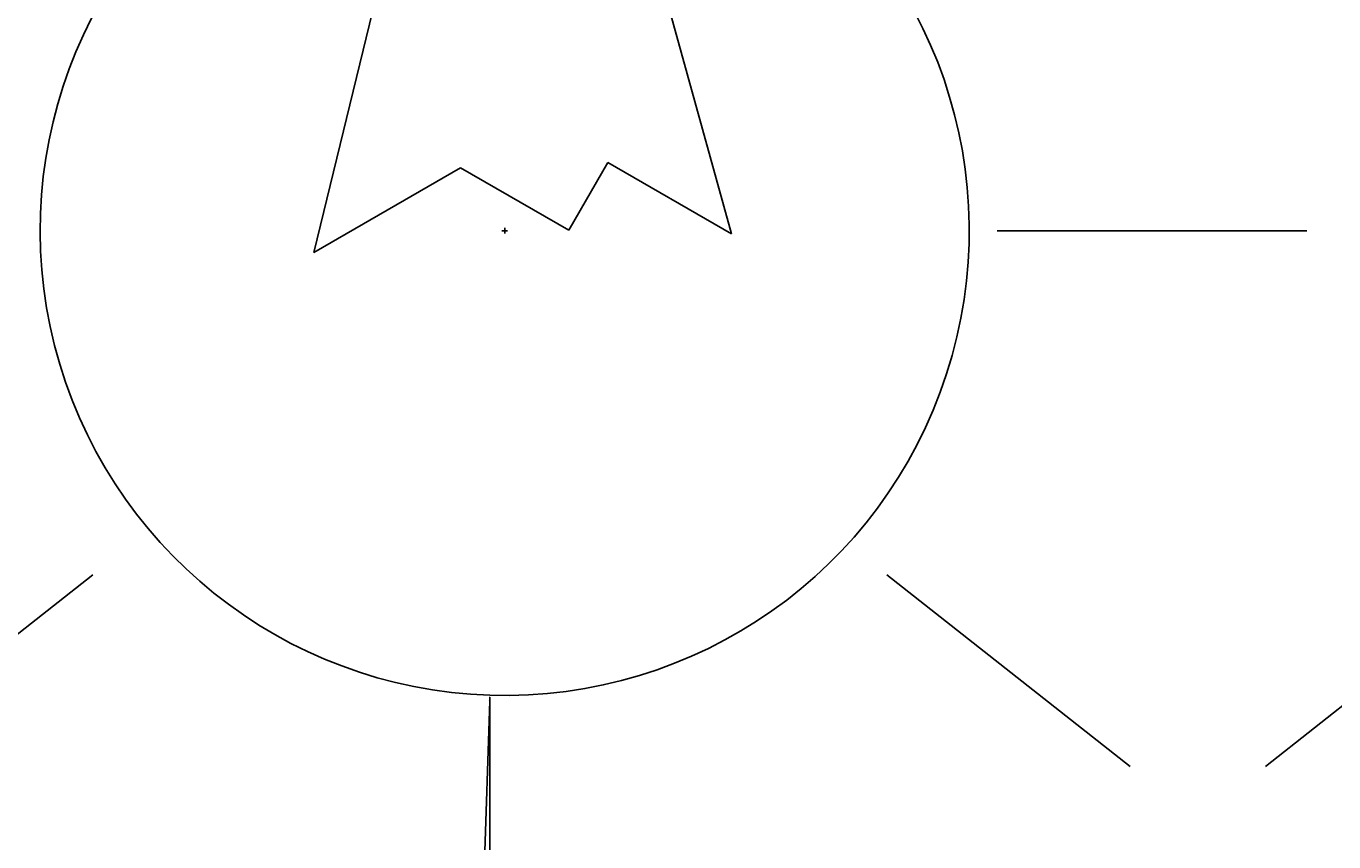
# Model space of a CAD drawing. Units: millimetres. Extents: x -8 to 285, y 5 to 221.
# Tile 23 of 30: x 130 to 172, y 132 to 159. Entities that reach past the tile are written whole.
import ezdxf

# ---------------------------------------------------------------- set-up
doc = ezdxf.new("R2010")
doc.units = ezdxf.units.MM
doc.layers.add('A-ANNO-DIMS', color=2, linetype='Continuous', lineweight=18)
doc.layers.add('E-LITE-FIXT', color=7, linetype='Continuous', lineweight=25)
doc.styles.get("Standard").update_dxf_attribs({"font": 'arial.ttf'})
doc.dimstyles.get("Standard").update_dxf_attribs({"dimtxt": 0.18, "dimasz": 0.18, "dimexe": 0.18, "dimexo": 0.0625, "dimgap": 0.09, "dimtad": 0, "dimtih": 1, "dimtoh": 1, "dimdec": 4, "dimzin": 0, "dimdsep": 46, "dimtxsty": 'Standard', "dimcen": 0.09, "dimadec": 0, "dimazin": 0, "dimtfac": 1, "dimtdec": 4, "dimtofl": 0, "dimtmove": 0, "dimatfit": 3, "dimfxl": 1, "dimtolj": 1, "dimtzin": 0, "dimarcsym": 0})

# ---------------------------------------------------------------- blocks, each defined once
blk = doc.blocks.new('LAMP-INCANDESCENT')
for p, q in [((7.407, 29.994), (10.595, 43.039)), ((23.407, 29.994), (18.595, 43.039)), ((9.734, 39.517), (19.894, 39.517)), ((9.001, 36.517), (21.001, 36.517)), ((8.268, 33.517), (22.107, 33.517)), ((7.407, 29.994), (7.407, 27.935)), ((12.666, 29.994), (8.834, 14.293)), ((22.321, 14.903), (18.146, 29.994)), ((23.407, 29.994), (23.407, 27.423)), ((8.834, 14.293), (13.574, 17.029)), ((13.574, 17.029), (17.067, 15.012)), ((17.067, 15.012), (18.333, 17.205)), ((18.333, 17.205), (22.321, 14.903))]:
    blk.add_line(p, q)
for points in [[(10.595, 43.039), (18.595, 43.039)], [(23.407, 29.994), (7.407, 29.994)]]:
    blk.add_lwpolyline(points)
for centre, radius, start, end in [((14.595, 43.039), 4, 0, 180), ((15.001, 15), 15, 88.4488, 91.5512), ((15.001, 15), 15, 120.4152, 55.9163)]:
    blk.add_arc(centre, radius, start, end)
blk = doc.blocks.new('*D9')
at = {"layer": 'A-ANNO-DIMS', "color": 0, "lineweight": -2, "transparency": 16777216}
for p, q in [((6.672, 133.79), (6.672, 220.737)), ((6.852, 220.557), (138.33, 220.557)), ((270.739, 220.557), (139.262, 220.557)), ((270.919, 206.519), (270.919, 220.737))]:
    blk.add_line(p, q, dxfattribs=at)
at = {"layer": 'A-ANNO-DIMS', "color": 0, "transparency": 16777216}
for points in [[(6.852, 220.587), (6.852, 220.527), (6.672, 220.557)], [(270.739, 220.587), (270.739, 220.527), (270.919, 220.557)]]:
    blk.add_solid(points, dxfattribs=at)
at = {"layer": 'Defpoints', "color": 0, "transparency": 16777216}
for p in [(270.919, 220.557), (270.919, 206.457), (6.672, 133.727)]:
    blk.add_point(p, dxfattribs=at)
at = {"layer": 'A-ANNO-DIMS', "color": 0, "transparency": 16777216, "insert": (138.796, 220.557), "char_height": 0.18, "attachment_point": 5}
blk.add_mtext('\\A1;264.25', dxfattribs=at)
blk = doc.blocks.new('*D10')
at = {"layer": 'A-ANNO-DIMS', "color": 0, "lineweight": -2, "transparency": 16777216}
for p, q in [((145.103, 206.457), (-7.608, 206.457)), ((-7.428, 206.277), (-7.428, 113.161)), ((-7.428, 19.682), (-7.428, 112.797)), ((30.453, 19.502), (-7.608, 19.502))]:
    blk.add_line(p, q, dxfattribs=at)
at = {"layer": 'A-ANNO-DIMS', "color": 0, "transparency": 16777216}
for points in [[(-7.458, 206.277), (-7.398, 206.277), (-7.428, 206.457)], [(-7.458, 19.682), (-7.398, 19.682), (-7.428, 19.502)]]:
    blk.add_solid(points, dxfattribs=at)
at = {"layer": 'Defpoints', "color": 0, "transparency": 16777216}
for p in [(-7.428, 206.457), (145.165, 206.457), (30.516, 19.502)]:
    blk.add_point(p, dxfattribs=at)
at = {"layer": 'A-ANNO-DIMS', "color": 0, "transparency": 16777216, "insert": (-7.428, 112.979), "char_height": 0.18, "attachment_point": 5}
blk.add_mtext('\\A1;186.95', dxfattribs=at)
blk = doc.blocks.new('*D13')
at = {"layer": 'A-ANNO-DIMS', "color": 0, "lineweight": -2, "transparency": 16777216}
for p, q in [((145.21, 137.013), (145.21, 5.222)), ((189.039, 137.013), (189.039, 5.222)), ((145.39, 5.402), (166.727, 5.402)), ((188.859, 5.402), (167.522, 5.402))]:
    blk.add_line(p, q, dxfattribs=at)
at = {"layer": 'A-ANNO-DIMS', "color": 0, "transparency": 16777216}
for points in [[(145.39, 5.432), (145.39, 5.372), (145.21, 5.402)], [(188.859, 5.432), (188.859, 5.372), (189.039, 5.402)]]:
    blk.add_solid(points, dxfattribs=at)
at = {"layer": 'Defpoints', "color": 0, "transparency": 16777216}
for p in [(145.21, 137.075), (189.039, 137.075), (189.039, 5.402)]:
    blk.add_point(p, dxfattribs=at)
at = {"layer": 'A-ANNO-DIMS', "color": 0, "transparency": 16777216, "insert": (167.124, 5.402), "char_height": 0.18, "attachment_point": 5}
blk.add_mtext('\\A1;43.83', dxfattribs=at)
blk = doc.blocks.new('*D29')
at = {"layer": 'A-ANNO-DIMS', "color": 0, "lineweight": -2, "transparency": 16777216}
for p, q in [((145.6, 152.068), (145.78, 152.068)), ((145.69, 151.978), (145.69, 152.158)), ((144.922, 128.08), (145.204, 136.895)), ((144.742, 128.08), (144.922, 128.08))]:
    blk.add_line(p, q, dxfattribs=at)
at = {"layer": 'A-ANNO-DIMS', "color": 0, "transparency": 16777216}
blk.add_solid([(145.174, 136.896), (145.234, 136.894), (145.21, 137.075)], dxfattribs=at)
at = {"layer": 'Defpoints', "color": 0, "transparency": 16777216}
for p in [(145.69, 152.068), (145.21, 137.075)]:
    blk.add_point(p, dxfattribs=at)
at = {"layer": 'A-ANNO-DIMS', "color": 0, "transparency": 16777216, "insert": (144.243, 128.08), "char_height": 0.18, "attachment_point": 5}
blk.add_mtext('\\A1;6X R15', dxfattribs=at)

msp = doc.modelspace()

# ---------------------------------------------------------------- linework, layer by layer
at = {"layer": 'E-LITE-FIXT'}
for p, q in [((171.5903, 152.0675), (161.5903, 152.0675)), ((132.3949, 140.9643), (124.5373, 134.7789)), ((158.0242, 140.9643), (165.8817, 134.7789)), ((178.1125, 140.9643), (170.2549, 134.7789))]:
    msp.add_line(p, q, dxfattribs=at)

# ---------------------------------------------------------------- block references
msp.add_blockref('LAMP-INCANDESCENT', (130.689, 137.068), dxfattribs=at)

# ---------------------------------------------------------------- dimensions: what is measured, and where the dimension line sits
at = {"layer": 'A-ANNO-DIMS'}
for base, p1, p2, picture, middle in [((270.9192, 220.5568), (6.6725, 133.7273), (270.9192, 206.4568), '*D9', (138.7958, 220.5568)), ((189.039, 5.402), (145.2095, 137.0752), (189.039, 137.0752), '*D13', (167.1243, 5.402))]:
    dim = msp.add_linear_dim(base=base, p1=p1, p2=p2, dimstyle='Standard', override={"dimdec": 2, "dimlfac": 1, "dimrnd": 0, "dimzin": 0, "dimdsep": 46, "dimlunit": 2}, dxfattribs=at)
    dim.commit()
    dim.dimension.update_dxf_attribs({"geometry": picture, "text_midpoint": middle})
dim = msp.add_linear_dim(base=(-7.4275, 206.4568), p1=(30.516, 19.502), p2=(145.1651, 206.4568), angle=90, dimstyle='Standard', override={"dimdec": 2, "dimlfac": 1, "dimrnd": 0, "dimzin": 0, "dimdsep": 46, "dimlunit": 2}, dxfattribs=at)
dim.commit()
dim.dimension.update_dxf_attribs({"geometry": '*D10', "text_midpoint": (-7.4275, 112.9794)})
dim = msp.add_radius_dim(center=(145.6897, 152.0675), mpoint=(145.21, 137.0752), text='6X <>', dimstyle='Standard', override={"dimdec": 0, "dimlfac": 1, "dimrnd": 0, "dimzin": 0, "dimdsep": 46, "dimlunit": 2}, dxfattribs=at)
dim.commit()
dim.dimension.update_dxf_attribs({"geometry": '*D29', "text_midpoint": (144.2426, 128.0798), "dimtype": 164})

doc.saveas('drawing.dxf')
